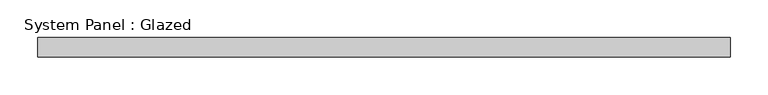
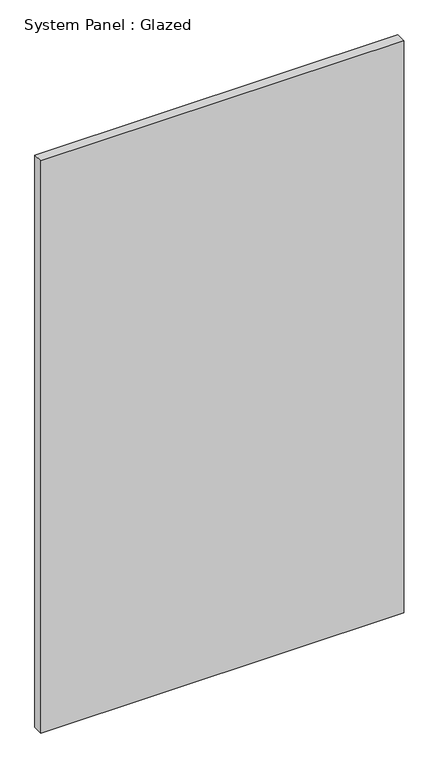
"""IFC4 building model written with IfcOpenShell, lengths in millimetres: plate geometry, System Panel : Glazed."""

from ifc_helpers import new_model, si_unit, origin, origin_with_axes, place, context, project, spatial, polyline, outline, extrude, source, transform, mapped, element, save


def system_panel_glazed_cdc09dc4(model_context):
    return source(origin(), model_context, "Body", "SweptSolid", [
        extrude(outline(polyline([(457.2, 19.05), (-457.2, 19.05), (-457.2, 44.45), (457.2, 44.45), (457.2, 19.05)])), origin_with_axes(), (0.0, 0.0, 1.0), 1524.0),
    ])


if __name__ == "__main__":
    model = new_model("IFC4")
    model_context = context("Model", 3, world=origin())
    ifc_project = project(units=[si_unit("LENGTHUNIT", "METRE", prefix="MILLI")], contexts=[model_context])
    site = spatial("IfcSite", under=ifc_project)
    building = spatial("IfcBuilding", under=site)
    placement = place(None, origin())
    system_panel_glazed_shape = system_panel_glazed_cdc09dc4(model_context)
    element("IfcPlate", 1, ObjectType="System Panel : Glazed", at=placement, inside=building, context=model_context, shape_type="MappedRepresentation", body=[
        mapped(system_panel_glazed_shape, transform((0.0, 0.0, 0.0), x_axis=(1.0, 0.0, 0.0), y_axis=(0.0, 1.0, 0.0), z_axis=(0.0, 0.0, 1.0))),
    ])
    save(model, "model.ifc")

# Revit data of these elements
# Type "System Panel : Glazed"
#   Construction Type Id = "GSP4R"
#   Analytic Construction = "1/8 in Pilkington single glazing"
#   Visual Light Transmittance = 0.9
#   Solar Heat Gain Coefficient = 0.86
#   Heat Transfer Coefficient (U) = 1.18115 BTU/(h·ft²·°F)
#   Define Thermal Properties by = 1
# Element 1 (IfcPlate, "System Panel : Glazed")
#   Materials on its faces: "Glass"
# Materials
#   "Glass": class "Glass", colour RGB 0 128 192, transparency 0.75, Description = "Soda Lime Glass", Cost = 0
